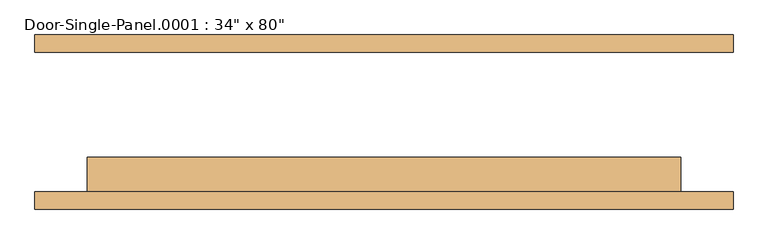
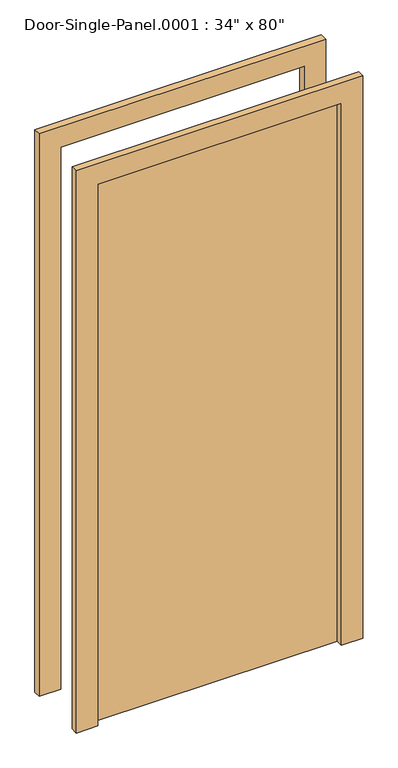
"""IFC4 building model written with IfcOpenShell, lengths in millimetres: door geometry."""

from ifc_helpers import new_model, si_unit, frame, origin, origin_with_axes, place, context, project, spatial, polyline, outline, extrude, source, transform, mapped, element, save


def door_2703ae13(model_context):
    return source(origin(), model_context, "Body", "SweptSolid", [
        extrude(outline(polyline([(431.8, -50.8), (431.8, -101.6), (-431.8, -101.6), (-431.8, -50.8), (431.8, -50.8)])), origin_with_axes(), (0.0, 0.0, 1.0), 2032.0),
        extrude(outline(polyline([(2108.2, -508.0), (0.0, -508.0), (0.0, -431.8), (2032.0, -431.8), (2032.0, 431.8), (0.0, 431.8), (0.0, 508.0), (2108.2, 508.0), (2108.2, -508.0)])), frame((0.0, -127.0, 0.0), z_axis=(0.0, 1.0, 0.0), x_axis=(0.0, 0.0, 1.0)), (0.0, 0.0, 1.0), 25.4),
        extrude(outline(polyline([(2108.2, 508.0), (2108.2, -508.0), (0.0, -508.0), (0.0, -431.8), (2032.0, -431.8), (2032.0, 431.8), (0.0, 431.8), (0.0, 508.0), (2108.2, 508.0)])), frame((0.0, 101.6, 0.0), z_axis=(0.0, 1.0, 0.0), x_axis=(0.0, 0.0, 1.0)), (0.0, 0.0, 1.0), 25.4),
    ])


if __name__ == "__main__":
    model = new_model("IFC4")
    model_context = context("Model", 3, world=origin())
    ifc_project = project(units=[si_unit("LENGTHUNIT", "METRE", prefix="MILLI")], contexts=[model_context])
    site = spatial("IfcSite", under=ifc_project)
    building = spatial("IfcBuilding", under=site)
    placement = place(None, origin())
    door_shape = door_2703ae13(model_context)
    element("IfcDoor", 1, ObjectType="Door-Single-Panel.0001 : 34\" x 80\"", at=placement, inside=building, context=model_context, shape_type="MappedRepresentation", body=[
        mapped(door_shape, transform((0.0, 0.0, 0.0), x_axis=(1.0, 0.0, 0.0), y_axis=(0.0, 1.0, 0.0), z_axis=(0.0, 0.0, 1.0))),
    ])
    save(model, "model.ifc")

# Revit data of these elements
# Type "Door-Single-Panel.0001 : 34\" x 80\""
#   Type Mark = "9"
#   Construction Type Id = "DOOR"
#   Assembly Code = "C1020300"
#   Analytic Construction = "Wooden"
#   Thickness = 0' - 2"
#   Thermal Resistance (R) = 0.455703 (m²·K)/W
#   Swing Angle [instance default] = 90.00°
#   Heat Transfer Coefficient (U) = 2.19465 W/(m²·K)
#   Height = 6' - 8"
#   Trim Projection Ext = 0' - 1"
#   Trim Projection Int = 0' - 1"
#   Trim Width = 0' - 3"
#   Width = 2' - 10"
#   Panel Material = Wood - Birch - Solid Stained Light Low Gloss
#   Trim Material = Paint - Sienna
#   Visual Light Transmittance = 0
#   Solar Heat Gain Coefficient = 0
#   Function = (empty or 0)
#   Wall Closure = (empty or 0)
# Element 1 (IfcDoor, "Door-Single-Panel.0001 : 34\" x 80\"")
#   Materials on its faces: "Paint - Sienna", "Wood - Birch - Solid Stained Light Low Gloss"
# Materials
#   "Wood - Birch - Solid Stained Light Low Gloss": class "Wood", colour RGB 210 159 95, transparency 0, Cost = 0
#   "Paint - Sienna": colour RGB 118 70 51, transparency 0, Cost = 0
